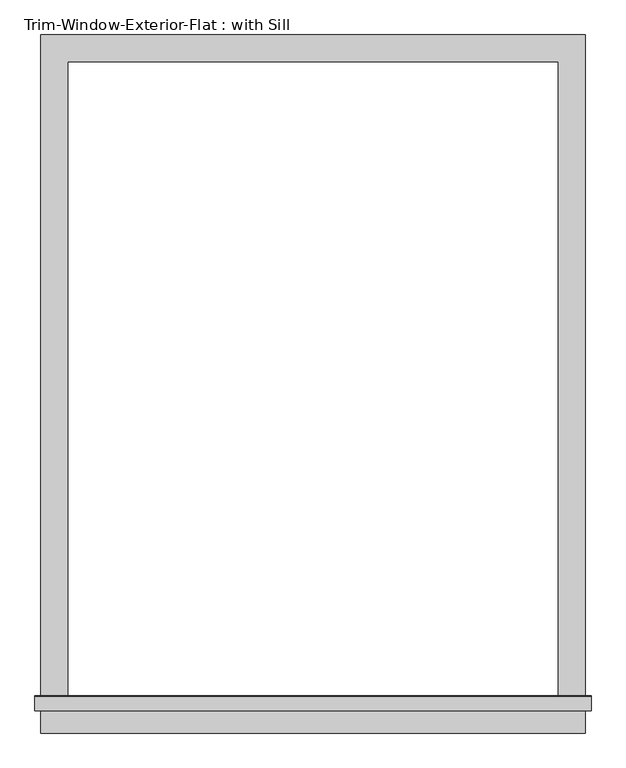
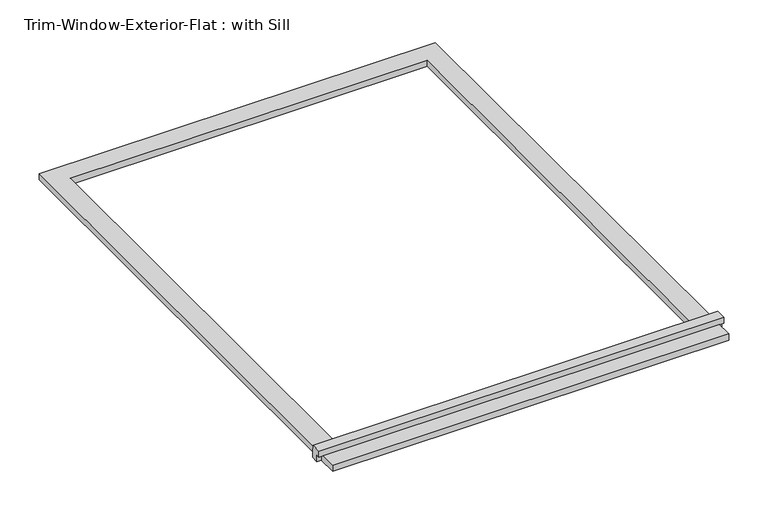
"""IFC4 building model written with IfcOpenShell, lengths in millimetres: proxy geometry, Trim-Window-Exterior-Flat : with Sill."""

from ifc_helpers import new_model, si_unit, frame, origin, origin_with_axes, place, context, project, spatial, polyline, outline, extrude, source, transform, mapped, element, save


def trim_window_exterior_flat_with_sill_4930676f(model_context):
    return source(origin(), model_context, "Body", "SweptSolid", [
        extrude(outline(polyline([(577.85, -1368.3823709), (577.85, -1425.5323709), (-577.85, -1425.5323709), (-577.85, -1368.3823709), (577.85, -1368.3823709)])), origin_with_axes(), (0.0, 0.0, 1.0), 19.05),
        extrude(outline(polyline([(-1377.95, 38.1), (-1348.6580645, 38.1), (-1346.2, 19.05), (-1346.2, 0.0), (-1368.3823709, 0.0), (-1368.3823709, 19.05), (-1377.95, 19.05), (-1377.95, 38.1)])), frame((-590.55, 0.0, 0.0), z_axis=(1.0, 0.0, 0.0), x_axis=(0.0, 1.0, 0.0)), (0.0, 0.0, 1.0), 1181.1),
        extrude(outline(polyline([(-577.85, 57.15), (577.85, 57.15), (577.85, -1346.2), (520.7, -1346.2), (520.7, 0.0), (-520.7, 0.0), (-520.7, -1346.2), (-577.85, -1346.2), (-577.85, 57.15)])), origin_with_axes(), (0.0, 0.0, 1.0), 19.05),
    ])


if __name__ == "__main__":
    model = new_model("IFC4")
    model_context = context("Model", 3, world=origin())
    ifc_project = project(units=[si_unit("LENGTHUNIT", "METRE", prefix="MILLI")], contexts=[model_context])
    site = spatial("IfcSite", under=ifc_project)
    building = spatial("IfcBuilding", under=site)
    placement = place(None, origin())
    trim_window_exterior_flat_with_sill_shape = trim_window_exterior_flat_with_sill_4930676f(model_context)
    element("IfcBuildingElementProxy", 1, Name="Trim-Window-Exterior-Flat : with Sill", ObjectType="Trim-Window-Exterior-Flat : with Sill", at=placement, inside=building, context=model_context, shape_type="MappedRepresentation", body=[
        mapped(trim_window_exterior_flat_with_sill_shape, transform((0.0, 0.0, 0.0), x_axis=(1.0, 0.0, 0.0), y_axis=(0.0, 1.0, 0.0), z_axis=(0.0, 0.0, 1.0))),
    ])
    save(model, "model.ifc")

# Revit data of these elements
# Type "Trim-Window-Exterior-Flat : with Sill"
#   Trim Width = 0' - 2 1/4"
#   Trim Thickness_Picture Frame = 0' - 1 1/4"
#   Trim Thickness_with Sill = 0' - 0 3/4"
#   Sill Thickness = 0' - 1 1/4"
#   Opening Width [instance default] = 2' - 0"
#   Opening Height [instance default] = 3' - 0"
#   Default Elevation = 4' - 0"
#   Sill = yes
#   Picture Frame = no
#   Trim Material [instance default] = none
# Element 1 (IfcBuildingElementProxy, "Trim-Window-Exterior-Flat : with Sill")
#   Opening Width = 3' - 5"
#   Opening Height = 4' - 5"
#   Trim Material = Clad - White
#   Materials on its faces: "Clad - White"
# Materials
#   "Clad - White": class "Wood", colour RGB 30 30 30, transparency 0, Cost = 0
